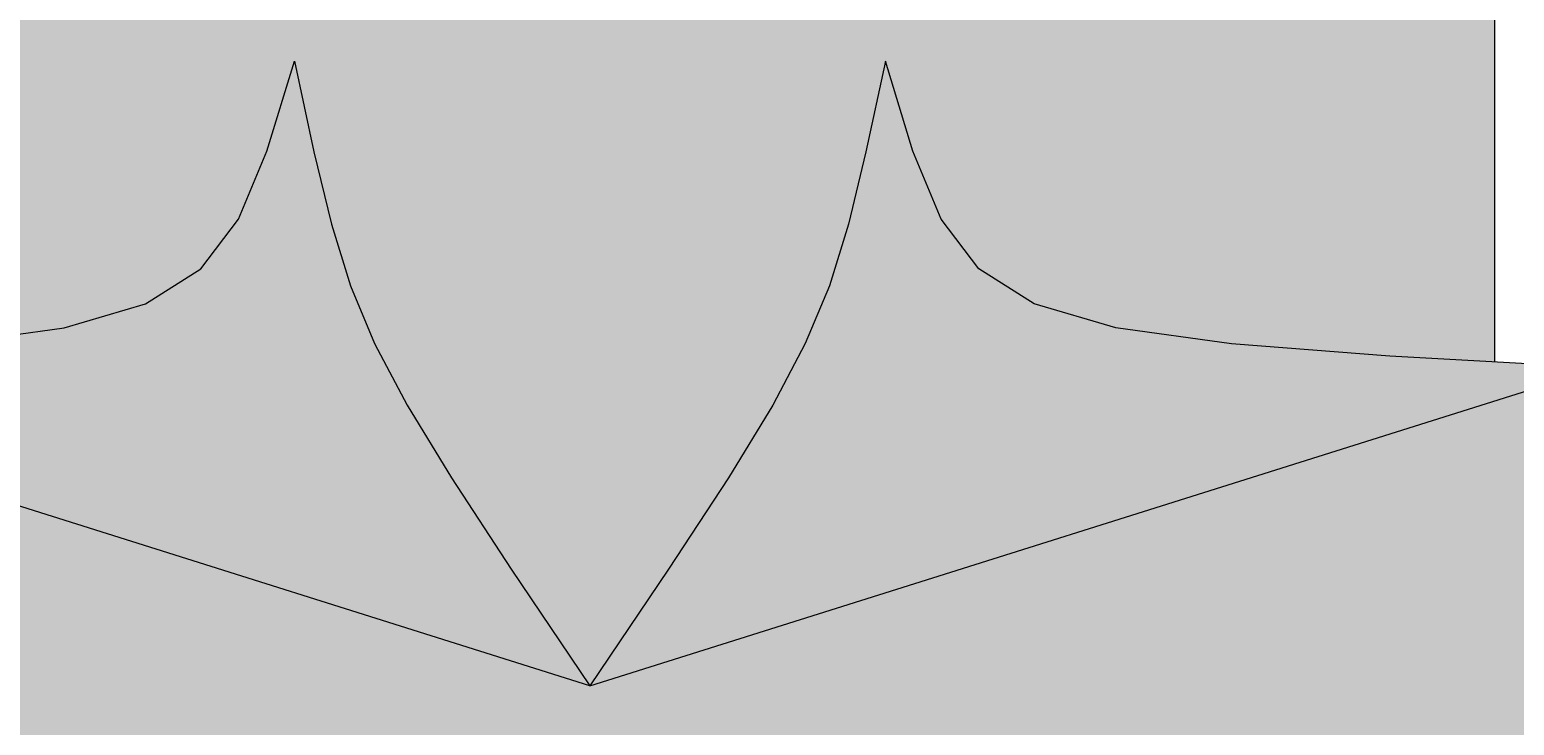
# Model space of a CAD drawing. Units: millimetres. Extents: x 27017497 to 27018854, y 7058029 to 7059154.
# Tile 75 of 91: x 27018390 to 27018436, y 7058163 to 7058185. Entities that reach past the tile are written whole.
import ezdxf

# ---------------------------------------------------------------- set-up
doc = ezdxf.new("R2010")
doc.units = ezdxf.units.MM
doc.layers.add('A-ANNO-DIMS', color=2, linetype='Continuous', lineweight=18)
doc.layers.add('A-FURN', color=8, linetype='Continuous', lineweight=18)
doc.layers.add('A-FURN-PATT', color=177, linetype='Continuous', lineweight=13, true_color=0x293189)
doc.styles.get("Standard").update_dxf_attribs({"font": 'arial.ttf'})
doc.dimstyles.get("Standard").update_dxf_attribs({"dimtxt": 0.18, "dimasz": 0.18, "dimexe": 0.18, "dimexo": 0.0625, "dimgap": 0.09, "dimtad": 0, "dimtih": 1, "dimtoh": 1, "dimdec": 4, "dimzin": 0, "dimdsep": 46, "dimtxsty": 'Standard', "dimcen": 0.09, "dimadec": 0, "dimazin": 0, "dimtfac": 1, "dimtdec": 4, "dimtofl": 0, "dimtmove": 0, "dimatfit": 3, "dimfxl": 1, "dimtolj": 1, "dimtzin": 0, "dimarcsym": 0})

# ---------------------------------------------------------------- blocks, each defined once
blk = doc.blocks.new('CAMMAT')
for p, q in [((0.0535, -0.5623), (-0.7312, -0.8093)), ((0.0535, -0.5623), (0.8382, -0.8093)), ((-0.65, -0.8139), (-0.65, -1.93))]:
    blk.add_line(p, q)
for points in [[(-0.1761, -1.0476), (-0.161, -0.9772), (-0.1474, -0.921), (-0.1326, -0.8732), (-0.1139, -0.8282), (-0.0886, -0.7803), (-0.0541, -0.7238), (-0.0076, -0.653), (0.0535, -0.5623)], [(0.2832, -1.0476), (0.2681, -0.9772), (0.2545, -0.921), (0.2396, -0.8732), (0.2209, -0.8282), (0.1957, -0.7803), (0.1611, -0.7238), (0.1147, -0.653), (0.0535, -0.5623)], [(-0.7312, -0.8093), (-0.5683, -0.8185), (-0.4451, -0.828), (-0.3552, -0.8406), (-0.2919, -0.8591), (-0.2489, -0.8862), (-0.2196, -0.9248), (-0.1975, -0.9777), (-0.1761, -1.0476)], [(0.8382, -0.8093), (0.6753, -0.8185), (0.5522, -0.828), (0.4622, -0.8406), (0.399, -0.8591), (0.356, -0.8862), (0.3267, -0.9248), (0.3046, -0.9777), (0.2832, -1.0476)]]:
    blk.add_lwpolyline(points)
blk = doc.blocks.new('*D47')
at = {"layer": 'A-ANNO-DIMS', "color": 0, "lineweight": -2, "transparency": 16777216}
for p, q in [((27017561.166, 7058294.35), (27017561.166, 7058028.6)), ((27018790.606, 7058294.35), (27018790.606, 7058028.6)), ((27017561.346, 7058028.78), (27018175.431, 7058028.78)), ((27018790.426, 7058028.78), (27018176.341, 7058028.78))]:
    blk.add_line(p, q, dxfattribs=at)
at = {"layer": 'A-ANNO-DIMS', "color": 0, "transparency": 16777216}
for points in [[(27017561.346, 7058028.81), (27017561.346, 7058028.75), (27017561.166, 7058028.78)], [(27018790.426, 7058028.81), (27018790.426, 7058028.75), (27018790.606, 7058028.78)]]:
    blk.add_solid(points, dxfattribs=at)
at = {"layer": 'Defpoints', "color": 0, "transparency": 16777216}
for p in [(27017561.166, 7058294.412), (27018790.606, 7058294.412), (27018790.606, 7058028.78)]:
    blk.add_point(p, dxfattribs=at)
at = {"layer": 'A-ANNO-DIMS', "color": 0, "transparency": 16777216, "insert": (27018175.886, 7058028.78), "char_height": 0.18, "attachment_point": 5}
blk.add_mtext('\\A1;1229.4', dxfattribs=at)
blk = doc.blocks.new('*D48')
at = {"layer": 'A-ANNO-DIMS', "color": 0, "lineweight": -2, "transparency": 16777216}
for p, q in [((27018463.498, 7058622.912), (27017497.536, 7058622.912)), ((27017497.716, 7058622.732), (27017497.716, 7058357.753)), ((27017497.716, 7058092.41), (27017497.716, 7058357.389)), ((27018555.129, 7058092.23), (27017497.536, 7058092.23))]:
    blk.add_line(p, q, dxfattribs=at)
at = {"layer": 'A-ANNO-DIMS', "color": 0, "transparency": 16777216}
for points in [[(27017497.686, 7058622.732), (27017497.746, 7058622.732), (27017497.716, 7058622.912)], [(27017497.686, 7058092.41), (27017497.746, 7058092.41), (27017497.716, 7058092.23)]]:
    blk.add_solid(points, dxfattribs=at)
at = {"layer": 'Defpoints', "color": 0, "transparency": 16777216}
for p in [(27018463.561, 7058622.912), (27017497.716, 7058092.23), (27018555.192, 7058092.23)]:
    blk.add_point(p, dxfattribs=at)
at = {"layer": 'A-ANNO-DIMS', "color": 0, "transparency": 16777216, "insert": (27017497.716, 7058357.571), "char_height": 0.18, "attachment_point": 5}
blk.add_mtext('\\A1;530.7', dxfattribs=at)

msp = doc.modelspace()

# ---------------------------------------------------------------- hatches: boundary and pattern name
at = {"layer": 'A-FURN-PATT'}
h = msp.add_hatch(color=256, dxfattribs=at)
h.dxf.hatch_style = 1
h.paths.add_polyline_path([(27018435.86, 7058218.784, 0.414214), (27018434.267, 7058220.377), (27018385.674, 7058220.377, 0.414214), (27018384.081, 7058218.784), (27018384.081, 7058174.59), (27018387.977, 7058174.891), (27018391.56, 7058175.393), (27018394.078, 7058176.128), (27018395.791, 7058177.21), (27018396.958, 7058178.748), (27018397.838, 7058180.854), (27018398.69, 7058183.639), (27018399.293, 7058180.835), (27018399.836, 7058178.594), (27018400.426, 7058176.691), (27018401.17, 7058174.899), (27018402.177, 7058172.991), (27018403.552, 7058170.741), (27018405.403, 7058167.922), (27018407.838, 7058164.308), (27018410.273, 7058167.922), (27018412.124, 7058170.741), (27018413.499, 7058172.991), (27018414.506, 7058174.899), (27018415.25, 7058176.691), (27018415.84, 7058178.594), (27018416.383, 7058180.835), (27018416.986, 7058183.639), (27018417.838, 7058180.854), (27018418.718, 7058178.748), (27018419.885, 7058177.21), (27018421.598, 7058176.128), (27018424.116, 7058175.393), (27018427.699, 7058174.891), (27018432.604, 7058174.513), (27018435.86, 7058174.329)])
h.paths.add_polyline_path([(27018439.093, 7058174.146), (27018432.604, 7058174.513), (27018427.699, 7058174.891), (27018424.116, 7058175.393), (27018421.598, 7058176.128), (27018419.885, 7058177.21), (27018418.718, 7058178.748), (27018417.838, 7058180.854), (27018416.986, 7058183.639), (27018416.383, 7058180.835), (27018415.84, 7058178.594), (27018415.25, 7058176.691), (27018414.506, 7058174.899), (27018413.499, 7058172.991), (27018412.124, 7058170.741), (27018410.273, 7058167.922), (27018407.838, 7058164.308)])
h.paths.add_polyline_path([(27018403.552, 7058170.741), (27018402.177, 7058172.991), (27018401.17, 7058174.899), (27018400.426, 7058176.691), (27018399.836, 7058178.594), (27018399.293, 7058180.835), (27018398.69, 7058183.639), (27018397.838, 7058180.854), (27018396.958, 7058178.748), (27018395.791, 7058177.21), (27018394.078, 7058176.128), (27018391.56, 7058175.393), (27018387.977, 7058174.891), (27018383.071, 7058174.513), (27018376.583, 7058174.146), (27018407.838, 7058164.308), (27018405.403, 7058167.922)])
h.paths.add_polyline_path([(27018437.469, 7058173.635), (27018407.838, 7058164.308), (27018382.784, 7058172.194), (27018382.784, 7058162.502), (27018437.469, 7058162.502)])
h.paths.add_polyline_path([(27018435.86, 7058162.502), (27018384.081, 7058162.502), (27018384.081, 7058146.294, 0.414214), (27018385.674, 7058144.7), (27018434.267, 7058144.7, 0.414214), (27018435.86, 7058146.294)])
h.paths.add_polyline_path([(27018407.684, 7058159.418, -0.41419), (27018408.879, 7058158.223), (27018408.879, 7058148.664, -0.414237), (27018407.684, 7058147.469), (27018386.224, 7058147.469, -0.41419), (27018385.029, 7058148.663), (27018385.029, 7058158.223, -0.414237), (27018386.224, 7058159.418)], flags=16)
h.paths.add_polyline_path([(27018411.821, 7058159.418), (27018433.28, 7058159.418, -0.41419), (27018434.475, 7058158.223), (27018434.475, 7058148.664, -0.414237), (27018433.28, 7058147.469), (27018411.821, 7058147.469, -0.414214), (27018410.626, 7058148.664), (27018410.626, 7058158.223, -0.414214)], flags=16)
h.paths.add_polyline_path([(27018382.886, 7058160.632), (27018362.971, 7058160.632), (27018362.971, 7058144.7), (27018382.886, 7058144.7)])
h.paths.add_polyline_path([(27018379.136, 7058152.033, -1), (27018367.187, 7058152.033, -1)], flags=16)
h.paths.add_polyline_path([(27018376.861, 7058152.033, -1), (27018369.461, 7058152.033, -1)], flags=0)
h.paths.add_polyline_path([(27018456.97, 7058160.632), (27018437.055, 7058160.632), (27018437.055, 7058144.7), (27018456.97, 7058144.7)])
h.paths.add_polyline_path([(27018453.028, 7058152.033, -1), (27018441.079, 7058152.033, -1)], flags=16)
h.paths.add_polyline_path([(27018450.754, 7058152.033, -1), (27018443.354, 7058152.033, -1)], flags=0)
h.paths.add_polyline_path([(27018434.475, 7058158.223, 0.41419), (27018433.28, 7058159.418), (27018411.821, 7058159.418, 0.414214), (27018410.626, 7058158.223), (27018410.626, 7058148.664, 0.414214), (27018411.821, 7058147.469), (27018433.28, 7058147.469, 0.414237), (27018434.475, 7058148.664)], flags=0)

# ---------------------------------------------------------------- block references
at = {"layer": 'A-FURN', "xscale": 39.82996475819422, "yscale": 39.82996475819422, "zscale": 39.82996475819422, "rotation": 180}
msp.add_blockref('CAMMAT', (27018409.97, 7058141.912), dxfattribs=at)

# ---------------------------------------------------------------- dimensions: what is measured, and where the dimension line sits
at = {"layer": 'A-ANNO-DIMS'}
dim = msp.add_linear_dim(base=(27017497.716, 7058092.23), p1=(27018463.561, 7058622.912), p2=(27018555.192, 7058092.23), angle=90, dimstyle='Standard', override={"dimdec": 1, "dimlfac": 1, "dimrnd": 0, "dimzin": 0, "dimdsep": 46, "dimlunit": 2}, dxfattribs=at)
dim.commit()
dim.dimension.update_dxf_attribs({"geometry": '*D48', "text_midpoint": (27017497.716, 7058357.571)})
dim = msp.add_linear_dim(base=(27018790.606, 7058028.78), p1=(27017561.166, 7058294.412), p2=(27018790.606, 7058294.412), dimstyle='Standard', override={"dimdec": 1, "dimlfac": 1, "dimrnd": 0, "dimzin": 0, "dimdsep": 46, "dimlunit": 2}, dxfattribs=at)
dim.commit()
dim.dimension.update_dxf_attribs({"geometry": '*D47', "text_midpoint": (27018175.886, 7058028.78)})

doc.saveas('drawing.dxf')
